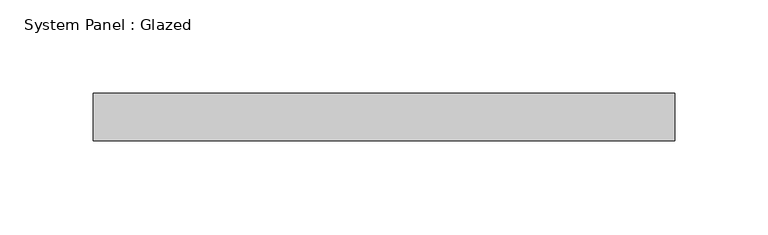
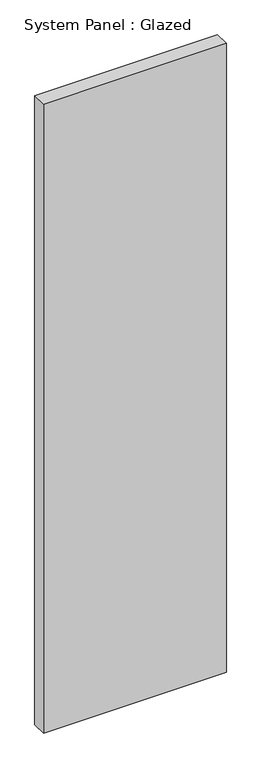
"""IFC4 building model written with IfcOpenShell, lengths in millimetres: plate geometry, System Panel : Glazed."""

from ifc_helpers import new_model, si_unit, origin, origin_with_axes, place, context, project, spatial, polyline, outline, extrude, source, transform, mapped, element, save


def system_panel_glazed_0848ed2a(model_context):
    return source(origin(), model_context, "Body", "SweptSolid", [
        extrude(outline(polyline([(155.575, 19.05), (-155.575, 19.05), (-155.575, 44.45), (155.575, 44.45), (155.575, 19.05)])), origin_with_axes(), (0.0, 0.0, 1.0), 1130.6019988),
    ])


if __name__ == "__main__":
    model = new_model("IFC4")
    model_context = context("Model", 3, world=origin())
    ifc_project = project(units=[si_unit("LENGTHUNIT", "METRE", prefix="MILLI")], contexts=[model_context])
    site = spatial("IfcSite", under=ifc_project)
    building = spatial("IfcBuilding", under=site)
    placement = place(None, origin())
    system_panel_glazed_shape = system_panel_glazed_0848ed2a(model_context)
    element("IfcPlate", 1, ObjectType="System Panel : Glazed", at=placement, inside=building, context=model_context, shape_type="MappedRepresentation", body=[
        mapped(system_panel_glazed_shape, transform((0.0, 0.0, 0.0), x_axis=(1.0, 0.0, 0.0), y_axis=(0.0, 1.0, 0.0), z_axis=(0.0, 0.0, 1.0))),
    ])
    save(model, "model.ifc")

# Revit data of these elements
# Type "System Panel : Glazed"
#   Construction Type Id = "GSP4R"
#   Analytic Construction = "1/8 in Pilkington single glazing"
#   Visual Light Transmittance = 0.9
#   Solar Heat Gain Coefficient = 0.86
#   Heat Transfer Coefficient (U) = 1.18115 BTU/(h·ft²·°F)
# Element 1 (IfcPlate, "System Panel : Glazed")
#   Materials on its faces: "Glass"
# Materials
#   "Glass": class "Glass", colour RGB 0 128 192, transparency 0.75, Description = "Soda Lime Glass", Cost = 0
